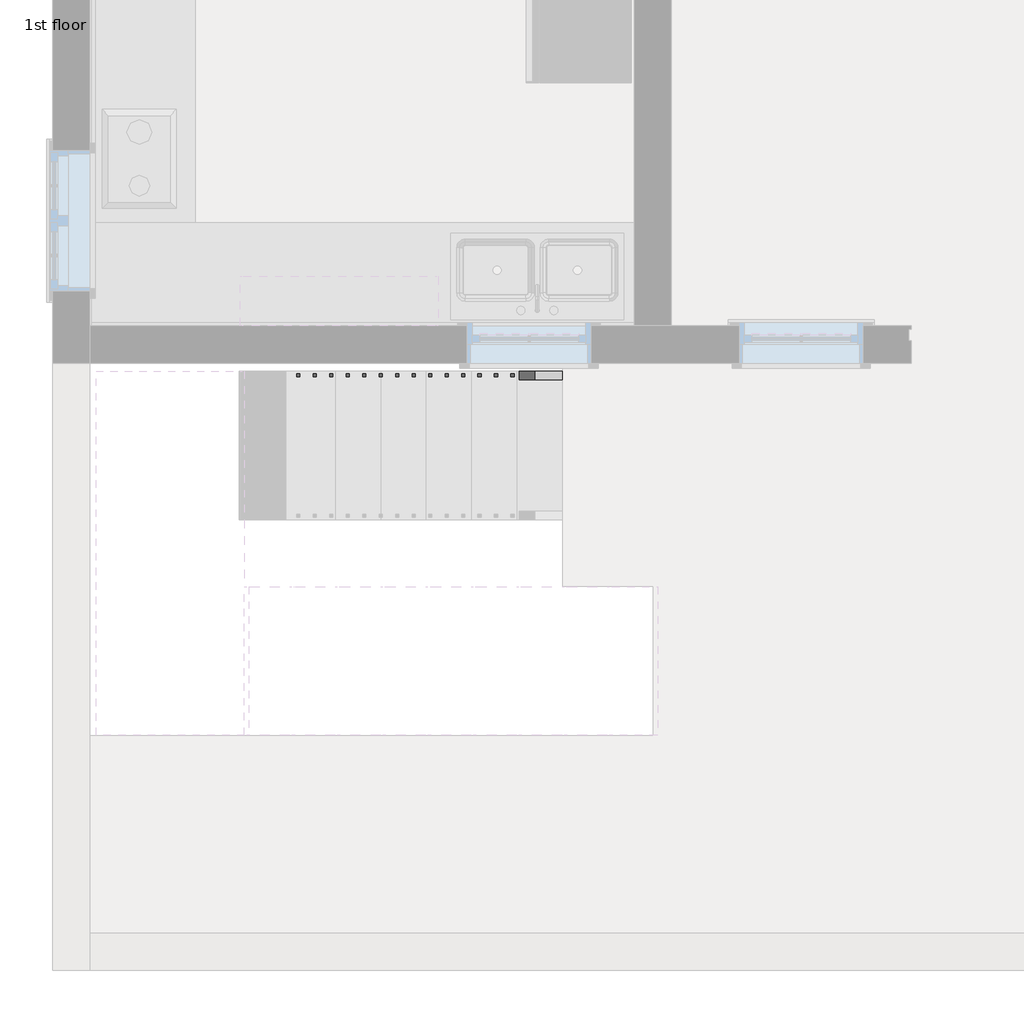
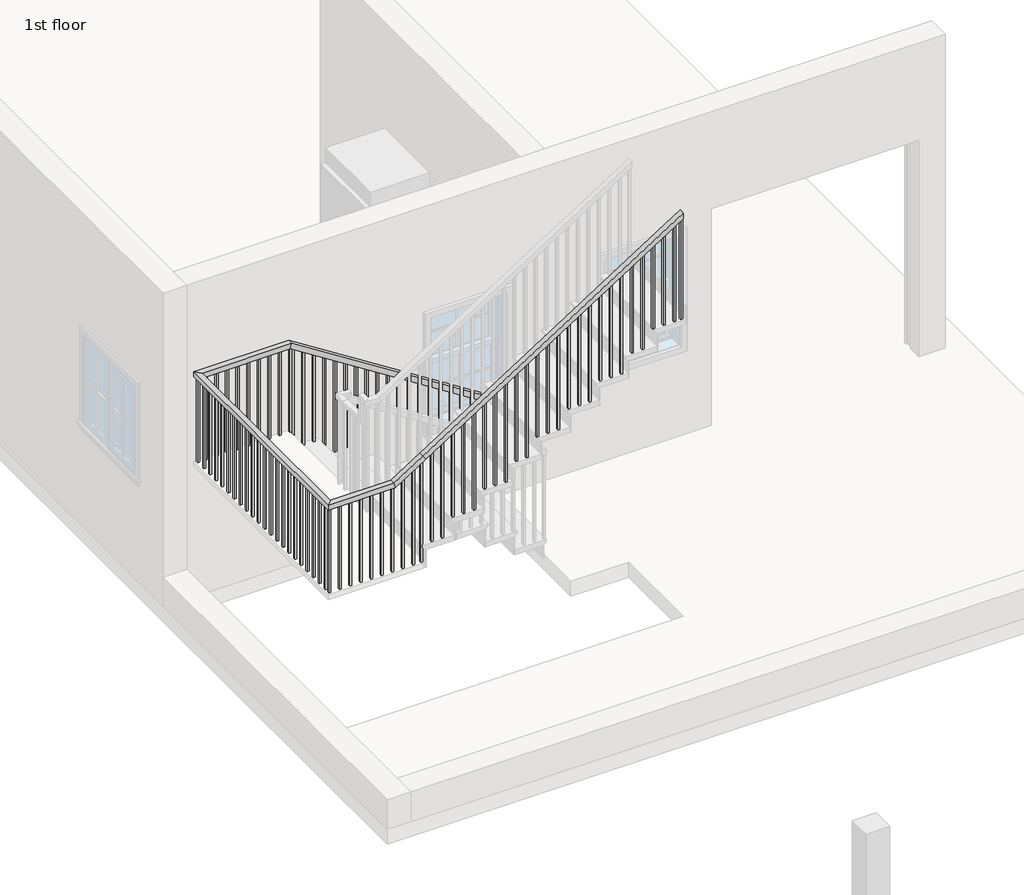
# One storey, part 2 of 3: 1 railing.
"""IFC4 building model written with IfcOpenShell, lengths in millimetres."""

from ifc_helpers import new_model, si_unit, frame, origin, place, context, project, spatial, polyline, outline, extrude, faceted_brep, element, save

model = new_model("IFC4")

# Units and contexts
model_context = context("Model", 3, world=origin())
ifc_project = project(units=[si_unit("LENGTHUNIT", "METRE", prefix="MILLI")], contexts=[model_context])

# Site, building, storey
site = spatial("IfcSite", under=ifc_project)
building = spatial("IfcBuilding", under=site)
storey = spatial("IfcBuildingStorey", under=building, Name="1st floor", Elevation=3810.0)

# Railing
placement = place(None, origin())
element("IfcRailing", 1, ObjectType="Handrail - Rectangular", at=placement, inside=storey, context=model_context, shape_type="SolidModel", body=[
    faceted_brep([(31519.2316163, 9231.5980552, 4902.2), (31519.2316163, 9231.5980552, 4841.986276), (31519.2316163, 9282.3980552, 4841.986276), (31519.2316163, 9282.3980552, 4902.2), (29563.4316163, 9231.5980552, 6146.8), (29548.6386214, 9231.5980552, 6096.0), (29548.6386214, 9282.3980552, 6096.0), (29563.4316163, 9282.3980552, 6146.8), (28699.8316163, 9231.5980552, 6146.8), (28699.8316163, 9231.5980552, 6096.0), (28649.0316163, 9282.3980552, 6096.0), (28649.0316163, 9282.3980552, 6146.8), (28699.8316163, 7091.6480552, 6146.8), (28699.8316163, 7091.6480552, 6096.0), (28649.0316163, 7040.8480552, 6096.0), (28649.0316163, 7040.8480552, 6146.8), (29284.0316163, 7091.6480552, 6146.8), (29298.8246113, 7091.6480552, 6096.0), (29298.8246113, 7040.8480552, 6096.0), (29284.0316163, 7040.8480552, 6146.8), (29563.4316163, 7091.6480552, 6324.6), (29590.7048913, 7091.6480552, 6281.7419964), (29590.7048913, 7040.8480552, 6281.7419964), (29563.4316163, 7040.8480552, 6324.6), (32078.0316163, 7091.6480552, 7924.8), (32078.0316163, 7040.8480552, 7924.8), (32078.0316163, 7040.8480552, 7864.586276), (32078.0316163, 7091.6480552, 7864.586276)], [[[0, 1, 2, 3]], [[1, 0, 4, 5]], [[2, 1, 5, 6]], [[3, 2, 6, 7]], [[0, 3, 7, 4]], [[5, 4, 8, 9]], [[6, 5, 9, 10]], [[7, 6, 10, 11]], [[4, 7, 11, 8]], [[9, 8, 12, 13]], [[10, 9, 13, 14]], [[11, 10, 14, 15]], [[8, 11, 15, 12]], [[13, 12, 16, 17]], [[14, 13, 17, 18]], [[15, 14, 18, 19]], [[12, 15, 19, 16]], [[17, 16, 20, 21]], [[18, 17, 21, 22]], [[19, 18, 22, 23]], [[16, 19, 23, 20]], [[24, 25, 26, 27]], [[21, 20, 24, 27]], [[22, 21, 27, 26]], [[23, 22, 26, 25]], [[20, 23, 25, 24]]]),
    extrude(outline(polyline([(7822.1567305, 32011.3566163), (7810.0340032, 31992.3066163), (6832.6, 31992.3066163), (6832.6, 32011.3566163), (7822.1567305, 32011.3566163)])), frame((0.0, 7056.7230552, 0.0), z_axis=(0.0, 1.0, 0.0), x_axis=(0.0, 0.0, 1.0)), (0.0, 0.0, 1.0), 19.05),
    extrude(outline(polyline([(7757.5021851, 31909.7566163), (7745.3794578, 31890.7066163), (6832.6, 31890.7066163), (6832.6, 31909.7566163), (7757.5021851, 31909.7566163)])), frame((0.0, 7056.7230552, 0.0), z_axis=(0.0, 1.0, 0.0), x_axis=(0.0, 0.0, 1.0)), (0.0, 0.0, 1.0), 19.05),
    extrude(outline(polyline([(7692.8476396, 31808.1566163), (7680.7249123, 31789.1066163), (6832.6, 31789.1066163), (6832.6, 31808.1566163), (7692.8476396, 31808.1566163)])), frame((0.0, 7056.7230552, 0.0), z_axis=(0.0, 1.0, 0.0), x_axis=(0.0, 0.0, 1.0)), (0.0, 0.0, 1.0), 19.05),
    extrude(outline(polyline([(7628.1930941, 31706.5566163), (7616.0703669, 31687.5066163), (6654.8, 31687.5066163), (6654.8, 31706.5566163), (7628.1930941, 31706.5566163)])), frame((0.0, 7056.7230552, 0.0), z_axis=(0.0, 1.0, 0.0), x_axis=(0.0, 0.0, 1.0)), (0.0, 0.0, 1.0), 19.05),
    extrude(outline(polyline([(7563.5385487, 31604.9566163), (7551.4158214, 31585.9066163), (6654.8, 31585.9066163), (6654.8, 31604.9566163), (7563.5385487, 31604.9566163)])), frame((0.0, 7056.7230552, 0.0), z_axis=(0.0, 1.0, 0.0), x_axis=(0.0, 0.0, 1.0)), (0.0, 0.0, 1.0), 19.05),
    extrude(outline(polyline([(7498.8840032, 31503.3566163), (7486.761276, 31484.3066163), (6477.0, 31484.3066163), (6477.0, 31503.3566163), (7498.8840032, 31503.3566163)])), frame((0.0, 7056.7230552, 0.0), z_axis=(0.0, 1.0, 0.0), x_axis=(0.0, 0.0, 1.0)), (0.0, 0.0, 1.0), 19.05),
    extrude(outline(polyline([(7434.2294578, 31401.7566163), (7422.1067305, 31382.7066163), (6477.0, 31382.7066163), (6477.0, 31401.7566163), (7434.2294578, 31401.7566163)])), frame((0.0, 7056.7230552, 0.0), z_axis=(0.0, 1.0, 0.0), x_axis=(0.0, 0.0, 1.0)), (0.0, 0.0, 1.0), 19.05),
    extrude(outline(polyline([(7369.5749123, 31300.1566163), (7357.4521851, 31281.1066163), (6477.0, 31281.1066163), (6477.0, 31300.1566163), (7369.5749123, 31300.1566163)])), frame((0.0, 7056.7230552, 0.0), z_axis=(0.0, 1.0, 0.0), x_axis=(0.0, 0.0, 1.0)), (0.0, 0.0, 1.0), 19.05),
    extrude(outline(polyline([(7304.9203669, 31198.5566163), (7292.7976396, 31179.5066163), (6299.2, 31179.5066163), (6299.2, 31198.5566163), (7304.9203669, 31198.5566163)])), frame((0.0, 7056.7230552, 0.0), z_axis=(0.0, 1.0, 0.0), x_axis=(0.0, 0.0, 1.0)), (0.0, 0.0, 1.0), 19.05),
    extrude(outline(polyline([(7240.2658214, 31096.9566163), (7228.1430941, 31077.9066163), (6299.2, 31077.9066163), (6299.2, 31096.9566163), (7240.2658214, 31096.9566163)])), frame((0.0, 7056.7230552, 0.0), z_axis=(0.0, 1.0, 0.0), x_axis=(0.0, 0.0, 1.0)), (0.0, 0.0, 1.0), 19.05),
    extrude(outline(polyline([(7175.611276, 30995.3566163), (7163.4885487, 30976.3066163), (6299.2, 30976.3066163), (6299.2, 30995.3566163), (7175.611276, 30995.3566163)])), frame((0.0, 7056.7230552, 0.0), z_axis=(0.0, 1.0, 0.0), x_axis=(0.0, 0.0, 1.0)), (0.0, 0.0, 1.0), 19.05),
    extrude(outline(polyline([(7110.9567305, 30893.7566163), (7098.8340032, 30874.7066163), (6121.4, 30874.7066163), (6121.4, 30893.7566163), (7110.9567305, 30893.7566163)])), frame((0.0, 7056.7230552, 0.0), z_axis=(0.0, 1.0, 0.0), x_axis=(0.0, 0.0, 1.0)), (0.0, 0.0, 1.0), 19.05),
    extrude(outline(polyline([(7046.3021851, 30792.1566163), (7034.1794578, 30773.1066163), (6121.4, 30773.1066163), (6121.4, 30792.1566163), (7046.3021851, 30792.1566163)])), frame((0.0, 7056.7230552, 0.0), z_axis=(0.0, 1.0, 0.0), x_axis=(0.0, 0.0, 1.0)), (0.0, 0.0, 1.0), 19.05),
    extrude(outline(polyline([(6981.6476396, 30690.5566163), (6969.5249123, 30671.5066163), (6121.4, 30671.5066163), (6121.4, 30690.5566163), (6981.6476396, 30690.5566163)])), frame((0.0, 7056.7230552, 0.0), z_axis=(0.0, 1.0, 0.0), x_axis=(0.0, 0.0, 1.0)), (0.0, 0.0, 1.0), 19.05),
    extrude(outline(polyline([(6916.9930941, 30588.9566163), (6904.8703669, 30569.9066163), (5943.6, 30569.9066163), (5943.6, 30588.9566163), (6916.9930941, 30588.9566163)])), frame((0.0, 7056.7230552, 0.0), z_axis=(0.0, 1.0, 0.0), x_axis=(0.0, 0.0, 1.0)), (0.0, 0.0, 1.0), 19.05),
    extrude(outline(polyline([(6852.3385487, 30487.3566163), (6840.2158214, 30468.3066163), (5943.6, 30468.3066163), (5943.6, 30487.3566163), (6852.3385487, 30487.3566163)])), frame((0.0, 7056.7230552, 0.0), z_axis=(0.0, 1.0, 0.0), x_axis=(0.0, 0.0, 1.0)), (0.0, 0.0, 1.0), 19.05),
    extrude(outline(polyline([(6787.6840032, 30385.7566163), (6775.561276, 30366.7066163), (5765.8, 30366.7066163), (5765.8, 30385.7566163), (6787.6840032, 30385.7566163)])), frame((0.0, 7056.7230552, 0.0), z_axis=(0.0, 1.0, 0.0), x_axis=(0.0, 0.0, 1.0)), (0.0, 0.0, 1.0), 19.05),
    extrude(outline(polyline([(6723.0294578, 30284.1566163), (6710.9067305, 30265.1066163), (5765.8, 30265.1066163), (5765.8, 30284.1566163), (6723.0294578, 30284.1566163)])), frame((0.0, 7056.7230552, 0.0), z_axis=(0.0, 1.0, 0.0), x_axis=(0.0, 0.0, 1.0)), (0.0, 0.0, 1.0), 19.05),
    extrude(outline(polyline([(6658.3749123, 30182.5566163), (6646.2521851, 30163.5066163), (5765.8, 30163.5066163), (5765.8, 30182.5566163), (6658.3749123, 30182.5566163)])), frame((0.0, 7056.7230552, 0.0), z_axis=(0.0, 1.0, 0.0), x_axis=(0.0, 0.0, 1.0)), (0.0, 0.0, 1.0), 19.05),
    extrude(outline(polyline([(6593.7203669, 30080.9566163), (6581.5976396, 30061.9066163), (5588.0, 30061.9066163), (5588.0, 30080.9566163), (6593.7203669, 30080.9566163)])), frame((0.0, 7056.7230552, 0.0), z_axis=(0.0, 1.0, 0.0), x_axis=(0.0, 0.0, 1.0)), (0.0, 0.0, 1.0), 19.05),
    extrude(outline(polyline([(6529.0658214, 29979.3566163), (6516.9430941, 29960.3066163), (5588.0, 29960.3066163), (5588.0, 29979.3566163), (6529.0658214, 29979.3566163)])), frame((0.0, 7056.7230552, 0.0), z_axis=(0.0, 1.0, 0.0), x_axis=(0.0, 0.0, 1.0)), (0.0, 0.0, 1.0), 19.05),
    extrude(outline(polyline([(6464.411276, 29877.7566163), (6452.2885487, 29858.7066163), (5588.0, 29858.7066163), (5588.0, 29877.7566163), (6464.411276, 29877.7566163)])), frame((0.0, 7056.7230552, 0.0), z_axis=(0.0, 1.0, 0.0), x_axis=(0.0, 0.0, 1.0)), (0.0, 0.0, 1.0), 19.05),
    extrude(outline(polyline([(6399.7567305, 29776.1566163), (6387.6340032, 29757.1066163), (5410.2, 29757.1066163), (5410.2, 29776.1566163), (6399.7567305, 29776.1566163)])), frame((0.0, 7056.7230552, 0.0), z_axis=(0.0, 1.0, 0.0), x_axis=(0.0, 0.0, 1.0)), (0.0, 0.0, 1.0), 19.05),
    extrude(outline(polyline([(6335.1021851, 29674.5566163), (6322.9794578, 29655.5066163), (5410.2, 29655.5066163), (5410.2, 29674.5566163), (6335.1021851, 29674.5566163)])), frame((0.0, 7056.7230552, 0.0), z_axis=(0.0, 1.0, 0.0), x_axis=(0.0, 0.0, 1.0)), (0.0, 0.0, 1.0), 19.05),
    extrude(outline(polyline([(6221.9567305, 29496.7566163), (6209.8340032, 29477.7066163), (5232.4, 29477.7066163), (5232.4, 29496.7566163), (6221.9567305, 29496.7566163)])), frame((0.0, 7056.7230552, 0.0), z_axis=(0.0, 1.0, 0.0), x_axis=(0.0, 0.0, 1.0)), (0.0, 0.0, 1.0), 19.05),
    extrude(outline(polyline([(6157.3021851, 29395.1566163), (6145.1794578, 29376.1066163), (5232.4, 29376.1066163), (5232.4, 29395.1566163), (6157.3021851, 29395.1566163)])), frame((0.0, 7056.7230552, 0.0), z_axis=(0.0, 1.0, 0.0), x_axis=(0.0, 0.0, 1.0)), (0.0, 0.0, 1.0), 19.05),
    extrude(outline(polyline([(29274.5066163, 7056.7230552), (29274.5066163, 7075.7730552), (29293.5566163, 7075.7730552), (29293.5566163, 7056.7230552), (29274.5066163, 7056.7230552)])), frame((0.0, 0.0, 5232.4), z_axis=(0.0, 0.0, 1.0), x_axis=(1.0, 0.0, 0.0)), (0.0, 0.0, 1.0), 863.6),
    extrude(outline(polyline([(29172.9066163, 7056.7230552), (29172.9066163, 7075.7730552), (29191.9566163, 7075.7730552), (29191.9566163, 7056.7230552), (29172.9066163, 7056.7230552)])), frame((0.0, 0.0, 5232.4), z_axis=(0.0, 0.0, 1.0), x_axis=(1.0, 0.0, 0.0)), (0.0, 0.0, 1.0), 863.6),
    extrude(outline(polyline([(29071.3066163, 7056.7230552), (29071.3066163, 7075.7730552), (29090.3566163, 7075.7730552), (29090.3566163, 7056.7230552), (29071.3066163, 7056.7230552)])), frame((0.0, 0.0, 5232.4), z_axis=(0.0, 0.0, 1.0), x_axis=(1.0, 0.0, 0.0)), (0.0, 0.0, 1.0), 863.6),
    extrude(outline(polyline([(28969.7066163, 7056.7230552), (28969.7066163, 7075.7730552), (28988.7566163, 7075.7730552), (28988.7566163, 7056.7230552), (28969.7066163, 7056.7230552)])), frame((0.0, 0.0, 5232.4), z_axis=(0.0, 0.0, 1.0), x_axis=(1.0, 0.0, 0.0)), (0.0, 0.0, 1.0), 863.6),
    extrude(outline(polyline([(28868.1066163, 7056.7230552), (28868.1066163, 7075.7730552), (28887.1566163, 7075.7730552), (28887.1566163, 7056.7230552), (28868.1066163, 7056.7230552)])), frame((0.0, 0.0, 5232.4), z_axis=(0.0, 0.0, 1.0), x_axis=(1.0, 0.0, 0.0)), (0.0, 0.0, 1.0), 863.6),
    extrude(outline(polyline([(28766.5066163, 7056.7230552), (28766.5066163, 7075.7730552), (28785.5566163, 7075.7730552), (28785.5566163, 7056.7230552), (28766.5066163, 7056.7230552)])), frame((0.0, 0.0, 5232.4), z_axis=(0.0, 0.0, 1.0), x_axis=(1.0, 0.0, 0.0)), (0.0, 0.0, 1.0), 863.6),
    extrude(outline(polyline([(28664.9066163, 7132.9230552), (28683.9566163, 7132.9230552), (28683.9566163, 7113.8730552), (28664.9066163, 7113.8730552), (28664.9066163, 7132.9230552)])), frame((0.0, 0.0, 5232.4), z_axis=(0.0, 0.0, 1.0), x_axis=(1.0, 0.0, 0.0)), (0.0, 0.0, 1.0), 863.6),
    extrude(outline(polyline([(28664.9066163, 7234.5230552), (28683.9566163, 7234.5230552), (28683.9566163, 7215.4730552), (28664.9066163, 7215.4730552), (28664.9066163, 7234.5230552)])), frame((0.0, 0.0, 5232.4), z_axis=(0.0, 0.0, 1.0), x_axis=(1.0, 0.0, 0.0)), (0.0, 0.0, 1.0), 863.6),
    extrude(outline(polyline([(28664.9066163, 7336.1230552), (28683.9566163, 7336.1230552), (28683.9566163, 7317.0730552), (28664.9066163, 7317.0730552), (28664.9066163, 7336.1230552)])), frame((0.0, 0.0, 5232.4), z_axis=(0.0, 0.0, 1.0), x_axis=(1.0, 0.0, 0.0)), (0.0, 0.0, 1.0), 863.6),
    extrude(outline(polyline([(28664.9066163, 7437.7230552), (28683.9566163, 7437.7230552), (28683.9566163, 7418.6730552), (28664.9066163, 7418.6730552), (28664.9066163, 7437.7230552)])), frame((0.0, 0.0, 5232.4), z_axis=(0.0, 0.0, 1.0), x_axis=(1.0, 0.0, 0.0)), (0.0, 0.0, 1.0), 863.6),
    extrude(outline(polyline([(28664.9066163, 7539.3230552), (28683.9566163, 7539.3230552), (28683.9566163, 7520.2730552), (28664.9066163, 7520.2730552), (28664.9066163, 7539.3230552)])), frame((0.0, 0.0, 5232.4), z_axis=(0.0, 0.0, 1.0), x_axis=(1.0, 0.0, 0.0)), (0.0, 0.0, 1.0), 863.6),
    extrude(outline(polyline([(28664.9066163, 7640.9230552), (28683.9566163, 7640.9230552), (28683.9566163, 7621.8730552), (28664.9066163, 7621.8730552), (28664.9066163, 7640.9230552)])), frame((0.0, 0.0, 5232.4), z_axis=(0.0, 0.0, 1.0), x_axis=(1.0, 0.0, 0.0)), (0.0, 0.0, 1.0), 863.6),
    extrude(outline(polyline([(28664.9066163, 7742.5230552), (28683.9566163, 7742.5230552), (28683.9566163, 7723.4730552), (28664.9066163, 7723.4730552), (28664.9066163, 7742.5230552)])), frame((0.0, 0.0, 5232.4), z_axis=(0.0, 0.0, 1.0), x_axis=(1.0, 0.0, 0.0)), (0.0, 0.0, 1.0), 863.6),
    extrude(outline(polyline([(28664.9066163, 7844.1230552), (28683.9566163, 7844.1230552), (28683.9566163, 7825.0730552), (28664.9066163, 7825.0730552), (28664.9066163, 7844.1230552)])), frame((0.0, 0.0, 5232.4), z_axis=(0.0, 0.0, 1.0), x_axis=(1.0, 0.0, 0.0)), (0.0, 0.0, 1.0), 863.6),
    extrude(outline(polyline([(28664.9066163, 7945.7230552), (28683.9566163, 7945.7230552), (28683.9566163, 7926.6730552), (28664.9066163, 7926.6730552), (28664.9066163, 7945.7230552)])), frame((0.0, 0.0, 5232.4), z_axis=(0.0, 0.0, 1.0), x_axis=(1.0, 0.0, 0.0)), (0.0, 0.0, 1.0), 863.6),
    extrude(outline(polyline([(28664.9066163, 8047.3230552), (28683.9566163, 8047.3230552), (28683.9566163, 8028.2730552), (28664.9066163, 8028.2730552), (28664.9066163, 8047.3230552)])), frame((0.0, 0.0, 5232.4), z_axis=(0.0, 0.0, 1.0), x_axis=(1.0, 0.0, 0.0)), (0.0, 0.0, 1.0), 863.6),
    extrude(outline(polyline([(28664.9066163, 8148.9230552), (28683.9566163, 8148.9230552), (28683.9566163, 8129.8730552), (28664.9066163, 8129.8730552), (28664.9066163, 8148.9230552)])), frame((0.0, 0.0, 5232.4), z_axis=(0.0, 0.0, 1.0), x_axis=(1.0, 0.0, 0.0)), (0.0, 0.0, 1.0), 863.6),
    extrude(outline(polyline([(28664.9066163, 8250.5230552), (28683.9566163, 8250.5230552), (28683.9566163, 8231.4730552), (28664.9066163, 8231.4730552), (28664.9066163, 8250.5230552)])), frame((0.0, 0.0, 5232.4), z_axis=(0.0, 0.0, 1.0), x_axis=(1.0, 0.0, 0.0)), (0.0, 0.0, 1.0), 863.6),
    extrude(outline(polyline([(28664.9066163, 8352.1230552), (28683.9566163, 8352.1230552), (28683.9566163, 8333.0730552), (28664.9066163, 8333.0730552), (28664.9066163, 8352.1230552)])), frame((0.0, 0.0, 5232.4), z_axis=(0.0, 0.0, 1.0), x_axis=(1.0, 0.0, 0.0)), (0.0, 0.0, 1.0), 863.6),
    extrude(outline(polyline([(28664.9066163, 8453.7230552), (28683.9566163, 8453.7230552), (28683.9566163, 8434.6730552), (28664.9066163, 8434.6730552), (28664.9066163, 8453.7230552)])), frame((0.0, 0.0, 5232.4), z_axis=(0.0, 0.0, 1.0), x_axis=(1.0, 0.0, 0.0)), (0.0, 0.0, 1.0), 863.6),
    extrude(outline(polyline([(28664.9066163, 8555.3230552), (28683.9566163, 8555.3230552), (28683.9566163, 8536.2730552), (28664.9066163, 8536.2730552), (28664.9066163, 8555.3230552)])), frame((0.0, 0.0, 5232.4), z_axis=(0.0, 0.0, 1.0), x_axis=(1.0, 0.0, 0.0)), (0.0, 0.0, 1.0), 863.6),
    extrude(outline(polyline([(28664.9066163, 8656.9230552), (28683.9566163, 8656.9230552), (28683.9566163, 8637.8730552), (28664.9066163, 8637.8730552), (28664.9066163, 8656.9230552)])), frame((0.0, 0.0, 5232.4), z_axis=(0.0, 0.0, 1.0), x_axis=(1.0, 0.0, 0.0)), (0.0, 0.0, 1.0), 863.6),
    extrude(outline(polyline([(28664.9066163, 8758.5230552), (28683.9566163, 8758.5230552), (28683.9566163, 8739.4730552), (28664.9066163, 8739.4730552), (28664.9066163, 8758.5230552)])), frame((0.0, 0.0, 5232.4), z_axis=(0.0, 0.0, 1.0), x_axis=(1.0, 0.0, 0.0)), (0.0, 0.0, 1.0), 863.6),
    extrude(outline(polyline([(28664.9066163, 8860.1230552), (28683.9566163, 8860.1230552), (28683.9566163, 8841.0730552), (28664.9066163, 8841.0730552), (28664.9066163, 8860.1230552)])), frame((0.0, 0.0, 5232.4), z_axis=(0.0, 0.0, 1.0), x_axis=(1.0, 0.0, 0.0)), (0.0, 0.0, 1.0), 863.6),
    extrude(outline(polyline([(28664.9066163, 8961.7230552), (28683.9566163, 8961.7230552), (28683.9566163, 8942.6730552), (28664.9066163, 8942.6730552), (28664.9066163, 8961.7230552)])), frame((0.0, 0.0, 5232.4), z_axis=(0.0, 0.0, 1.0), x_axis=(1.0, 0.0, 0.0)), (0.0, 0.0, 1.0), 863.6),
    extrude(outline(polyline([(28664.9066163, 9063.3230552), (28683.9566163, 9063.3230552), (28683.9566163, 9044.2730552), (28664.9066163, 9044.2730552), (28664.9066163, 9063.3230552)])), frame((0.0, 0.0, 5232.4), z_axis=(0.0, 0.0, 1.0), x_axis=(1.0, 0.0, 0.0)), (0.0, 0.0, 1.0), 863.6),
    extrude(outline(polyline([(28664.9066163, 9164.9230552), (28683.9566163, 9164.9230552), (28683.9566163, 9145.8730552), (28664.9066163, 9145.8730552), (28664.9066163, 9164.9230552)])), frame((0.0, 0.0, 5232.4), z_axis=(0.0, 0.0, 1.0), x_axis=(1.0, 0.0, 0.0)), (0.0, 0.0, 1.0), 863.6),
    extrude(outline(polyline([(28760.1566163, 9266.5230552), (28760.1566163, 9247.4730552), (28741.1066163, 9247.4730552), (28741.1066163, 9266.5230552), (28760.1566163, 9266.5230552)])), frame((0.0, 0.0, 5232.4), z_axis=(0.0, 0.0, 1.0), x_axis=(1.0, 0.0, 0.0)), (0.0, 0.0, 1.0), 863.6),
    extrude(outline(polyline([(28861.7566163, 9266.5230552), (28861.7566163, 9247.4730552), (28842.7066163, 9247.4730552), (28842.7066163, 9266.5230552), (28861.7566163, 9266.5230552)])), frame((0.0, 0.0, 5232.4), z_axis=(0.0, 0.0, 1.0), x_axis=(1.0, 0.0, 0.0)), (0.0, 0.0, 1.0), 863.6),
    extrude(outline(polyline([(28963.3566163, 9266.5230552), (28963.3566163, 9247.4730552), (28944.3066163, 9247.4730552), (28944.3066163, 9266.5230552), (28963.3566163, 9266.5230552)])), frame((0.0, 0.0, 5232.4), z_axis=(0.0, 0.0, 1.0), x_axis=(1.0, 0.0, 0.0)), (0.0, 0.0, 1.0), 863.6),
    extrude(outline(polyline([(29064.9566163, 9266.5230552), (29064.9566163, 9247.4730552), (29045.9066163, 9247.4730552), (29045.9066163, 9266.5230552), (29064.9566163, 9266.5230552)])), frame((0.0, 0.0, 5232.4), z_axis=(0.0, 0.0, 1.0), x_axis=(1.0, 0.0, 0.0)), (0.0, 0.0, 1.0), 863.6),
    extrude(outline(polyline([(29166.5566163, 9266.5230552), (29166.5566163, 9247.4730552), (29147.5066163, 9247.4730552), (29147.5066163, 9266.5230552), (29166.5566163, 9266.5230552)])), frame((0.0, 0.0, 5232.4), z_axis=(0.0, 0.0, 1.0), x_axis=(1.0, 0.0, 0.0)), (0.0, 0.0, 1.0), 863.6),
    extrude(outline(polyline([(29268.1566163, 9266.5230552), (29268.1566163, 9247.4730552), (29249.1066163, 9247.4730552), (29249.1066163, 9266.5230552), (29268.1566163, 9266.5230552)])), frame((0.0, 0.0, 5232.4), z_axis=(0.0, 0.0, 1.0), x_axis=(1.0, 0.0, 0.0)), (0.0, 0.0, 1.0), 863.6),
    extrude(outline(polyline([(29369.7566163, 9266.5230552), (29369.7566163, 9247.4730552), (29350.7066163, 9247.4730552), (29350.7066163, 9266.5230552), (29369.7566163, 9266.5230552)])), frame((0.0, 0.0, 5232.4), z_axis=(0.0, 0.0, 1.0), x_axis=(1.0, 0.0, 0.0)), (0.0, 0.0, 1.0), 863.6),
    extrude(outline(polyline([(29471.3566163, 9266.5230552), (29471.3566163, 9247.4730552), (29452.3066163, 9247.4730552), (29452.3066163, 9266.5230552), (29471.3566163, 9266.5230552)])), frame((0.0, 0.0, 5232.4), z_axis=(0.0, 0.0, 1.0), x_axis=(1.0, 0.0, 0.0)), (0.0, 0.0, 1.0), 863.6),
    extrude(outline(polyline([(6064.361276, 29598.3566163), (6076.4840032, 29579.3066163), (5054.6, 29579.3066163), (5054.6, 29598.3566163), (6064.361276, 29598.3566163)])), frame((0.0, 9247.4730552, 0.0), z_axis=(0.0, 1.0, 0.0), x_axis=(0.0, 0.0, 1.0)), (0.0, 0.0, 1.0), 19.05),
    extrude(outline(polyline([(5999.7067305, 29699.9566163), (6011.8294578, 29680.9066163), (5054.6, 29680.9066163), (5054.6, 29699.9566163), (5999.7067305, 29699.9566163)])), frame((0.0, 9247.4730552, 0.0), z_axis=(0.0, 1.0, 0.0), x_axis=(0.0, 0.0, 1.0)), (0.0, 0.0, 1.0), 19.05),
    extrude(outline(polyline([(5935.0521851, 29801.5566163), (5947.1749123, 29782.5066163), (5054.6, 29782.5066163), (5054.6, 29801.5566163), (5935.0521851, 29801.5566163)])), frame((0.0, 9247.4730552, 0.0), z_axis=(0.0, 1.0, 0.0), x_axis=(0.0, 0.0, 1.0)), (0.0, 0.0, 1.0), 19.05),
    extrude(outline(polyline([(5870.3976396, 29903.1566163), (5882.5203669, 29884.1066163), (4876.8, 29884.1066163), (4876.8, 29903.1566163), (5870.3976396, 29903.1566163)])), frame((0.0, 9247.4730552, 0.0), z_axis=(0.0, 1.0, 0.0), x_axis=(0.0, 0.0, 1.0)), (0.0, 0.0, 1.0), 19.05),
    extrude(outline(polyline([(5805.7430941, 30004.7566163), (5817.8658214, 29985.7066163), (4876.8, 29985.7066163), (4876.8, 30004.7566163), (5805.7430941, 30004.7566163)])), frame((0.0, 9247.4730552, 0.0), z_axis=(0.0, 1.0, 0.0), x_axis=(0.0, 0.0, 1.0)), (0.0, 0.0, 1.0), 19.05),
    extrude(outline(polyline([(5741.0885487, 30106.3566163), (5753.211276, 30087.3066163), (4876.8, 30087.3066163), (4876.8, 30106.3566163), (5741.0885487, 30106.3566163)])), frame((0.0, 9247.4730552, 0.0), z_axis=(0.0, 1.0, 0.0), x_axis=(0.0, 0.0, 1.0)), (0.0, 0.0, 1.0), 19.05),
    extrude(outline(polyline([(5676.4340032, 30207.9566163), (5688.5567305, 30188.9066163), (4699.0, 30188.9066163), (4699.0, 30207.9566163), (5676.4340032, 30207.9566163)])), frame((0.0, 9247.4730552, 0.0), z_axis=(0.0, 1.0, 0.0), x_axis=(0.0, 0.0, 1.0)), (0.0, 0.0, 1.0), 19.05),
    extrude(outline(polyline([(5611.7794578, 30309.5566163), (5623.9021851, 30290.5066163), (4699.0, 30290.5066163), (4699.0, 30309.5566163), (5611.7794578, 30309.5566163)])), frame((0.0, 9247.4730552, 0.0), z_axis=(0.0, 1.0, 0.0), x_axis=(0.0, 0.0, 1.0)), (0.0, 0.0, 1.0), 19.05),
    extrude(outline(polyline([(5547.1249123, 30411.1566163), (5559.2476396, 30392.1066163), (4699.0, 30392.1066163), (4699.0, 30411.1566163), (5547.1249123, 30411.1566163)])), frame((0.0, 9247.4730552, 0.0), z_axis=(0.0, 1.0, 0.0), x_axis=(0.0, 0.0, 1.0)), (0.0, 0.0, 1.0), 19.05),
    extrude(outline(polyline([(5482.4703669, 30512.7566163), (5494.5930941, 30493.7066163), (4521.2, 30493.7066163), (4521.2, 30512.7566163), (5482.4703669, 30512.7566163)])), frame((0.0, 9247.4730552, 0.0), z_axis=(0.0, 1.0, 0.0), x_axis=(0.0, 0.0, 1.0)), (0.0, 0.0, 1.0), 19.05),
    extrude(outline(polyline([(5417.8158214, 30614.3566163), (5429.9385487, 30595.3066163), (4521.2, 30595.3066163), (4521.2, 30614.3566163), (5417.8158214, 30614.3566163)])), frame((0.0, 9247.4730552, 0.0), z_axis=(0.0, 1.0, 0.0), x_axis=(0.0, 0.0, 1.0)), (0.0, 0.0, 1.0), 19.05),
    extrude(outline(polyline([(5353.161276, 30715.9566163), (5365.2840032, 30696.9066163), (4343.4, 30696.9066163), (4343.4, 30715.9566163), (5353.161276, 30715.9566163)])), frame((0.0, 9247.4730552, 0.0), z_axis=(0.0, 1.0, 0.0), x_axis=(0.0, 0.0, 1.0)), (0.0, 0.0, 1.0), 19.05),
    extrude(outline(polyline([(5288.5067305, 30817.5566163), (5300.6294578, 30798.5066163), (4343.4, 30798.5066163), (4343.4, 30817.5566163), (5288.5067305, 30817.5566163)])), frame((0.0, 9247.4730552, 0.0), z_axis=(0.0, 1.0, 0.0), x_axis=(0.0, 0.0, 1.0)), (0.0, 0.0, 1.0), 19.05),
    extrude(outline(polyline([(5223.8521851, 30919.1566163), (5235.9749123, 30900.1066163), (4343.4, 30900.1066163), (4343.4, 30919.1566163), (5223.8521851, 30919.1566163)])), frame((0.0, 9247.4730552, 0.0), z_axis=(0.0, 1.0, 0.0), x_axis=(0.0, 0.0, 1.0)), (0.0, 0.0, 1.0), 19.05),
    extrude(outline(polyline([(5159.1976396, 31020.7566163), (5171.3203669, 31001.7066163), (4165.6, 31001.7066163), (4165.6, 31020.7566163), (5159.1976396, 31020.7566163)])), frame((0.0, 9247.4730552, 0.0), z_axis=(0.0, 1.0, 0.0), x_axis=(0.0, 0.0, 1.0)), (0.0, 0.0, 1.0), 19.05),
    extrude(outline(polyline([(5094.5430941, 31122.3566163), (5106.6658214, 31103.3066163), (4165.6, 31103.3066163), (4165.6, 31122.3566163), (5094.5430941, 31122.3566163)])), frame((0.0, 9247.4730552, 0.0), z_axis=(0.0, 1.0, 0.0), x_axis=(0.0, 0.0, 1.0)), (0.0, 0.0, 1.0), 19.05),
    extrude(outline(polyline([(5029.8885487, 31223.9566163), (5042.011276, 31204.9066163), (4165.6, 31204.9066163), (4165.6, 31223.9566163), (5029.8885487, 31223.9566163)])), frame((0.0, 9247.4730552, 0.0), z_axis=(0.0, 1.0, 0.0), x_axis=(0.0, 0.0, 1.0)), (0.0, 0.0, 1.0), 19.05),
    extrude(outline(polyline([(4965.2340032, 31325.5566163), (4977.3567305, 31306.5066163), (3987.8, 31306.5066163), (3987.8, 31325.5566163), (4965.2340032, 31325.5566163)])), frame((0.0, 9247.4730552, 0.0), z_axis=(0.0, 1.0, 0.0), x_axis=(0.0, 0.0, 1.0)), (0.0, 0.0, 1.0), 19.05),
    extrude(outline(polyline([(4900.5794578, 31427.1566163), (4912.7021851, 31408.1066163), (3987.8, 31408.1066163), (3987.8, 31427.1566163), (4900.5794578, 31427.1566163)])), frame((0.0, 9247.4730552, 0.0), z_axis=(0.0, 1.0, 0.0), x_axis=(0.0, 0.0, 1.0)), (0.0, 0.0, 1.0), 19.05),
    extrude(outline(polyline([(6270.4476396, 29572.9566163), (6258.3249123, 29553.9066163), (5232.4, 29553.9066163), (5232.4, 29572.9566163), (6270.4476396, 29572.9566163)])), frame((0.0, 7056.7230552, 0.0), z_axis=(0.0, 1.0, 0.0), x_axis=(0.0, 0.0, 1.0)), (0.0, 0.0, 1.0), 19.05),
    extrude(outline(polyline([(28664.9066163, 7075.7730552), (28683.9566163, 7075.7730552), (28683.9566163, 7056.7230552), (28664.9066163, 7056.7230552), (28664.9066163, 7075.7730552)])), frame((0.0, 0.0, 5232.4), z_axis=(0.0, 0.0, 1.0), x_axis=(1.0, 0.0, 0.0)), (0.0, 0.0, 1.0), 863.6),
    extrude(outline(polyline([(28683.9566163, 9266.5230552), (28683.9566163, 9247.4730552), (28664.9066163, 9247.4730552), (28664.9066163, 9266.5230552), (28683.9566163, 9266.5230552)])), frame((0.0, 0.0, 5232.4), z_axis=(0.0, 0.0, 1.0), x_axis=(1.0, 0.0, 0.0)), (0.0, 0.0, 1.0), 863.6),
    extrude(outline(polyline([(6080.5249123, 29572.9566163), (6092.6476396, 29553.9066163), (5232.4, 29553.9066163), (5232.4, 29572.9566163), (6080.5249123, 29572.9566163)])), frame((0.0, 9247.4730552, 0.0), z_axis=(0.0, 1.0, 0.0), x_axis=(0.0, 0.0, 1.0)), (0.0, 0.0, 1.0), 19.05),
    extrude(outline(polyline([(7864.586276, 32078.0316163), (7852.4635487, 32058.9816163), (6832.6, 32058.9816163), (6832.6, 32078.0316163), (7864.586276, 32078.0316163)])), frame((0.0, 7056.7230552, 0.0), z_axis=(0.0, 1.0, 0.0), x_axis=(0.0, 0.0, 1.0)), (0.0, 0.0, 1.0), 19.05),
    extrude(outline(polyline([(4841.986276, 31519.2316163), (4854.1090032, 31500.1816163), (3987.8, 31500.1816163), (3987.8, 31519.2316163), (4841.986276, 31519.2316163)])), frame((0.0, 9247.4730552, 0.0), z_axis=(0.0, 1.0, 0.0), x_axis=(0.0, 0.0, 1.0)), (0.0, 0.0, 1.0), 19.05),
])

save(model, "model.ifc")

# Revit data of these elements
# Type "Handrail - Rectangular"
#   Assembly Code = "C2010400"
#   built-in parameter 1008612 = 0.0416667 (stored number, unit not read)
#   built-in parameter 1008611 = 0.0416667 (stored number, unit not read)
#   built-in parameter 1008609 = 0.333333 (stored number, unit not read)
#   built-in parameter 1008604 = 0.166667 (stored number, unit not read)
#   built-in parameter 1008603 = 0.166667 (stored number, unit not read)
#   Railing Height = 3' - 0"
#   built-in parameter 1008630 = 2
#   built-in parameter 1008610 = 2
#   built-in parameter 1008618 = Baluster - Square : 3/4"
# Element 1 (IfcRailing, "Handrail - Rectangular")
#   Phase Created = New Construction
